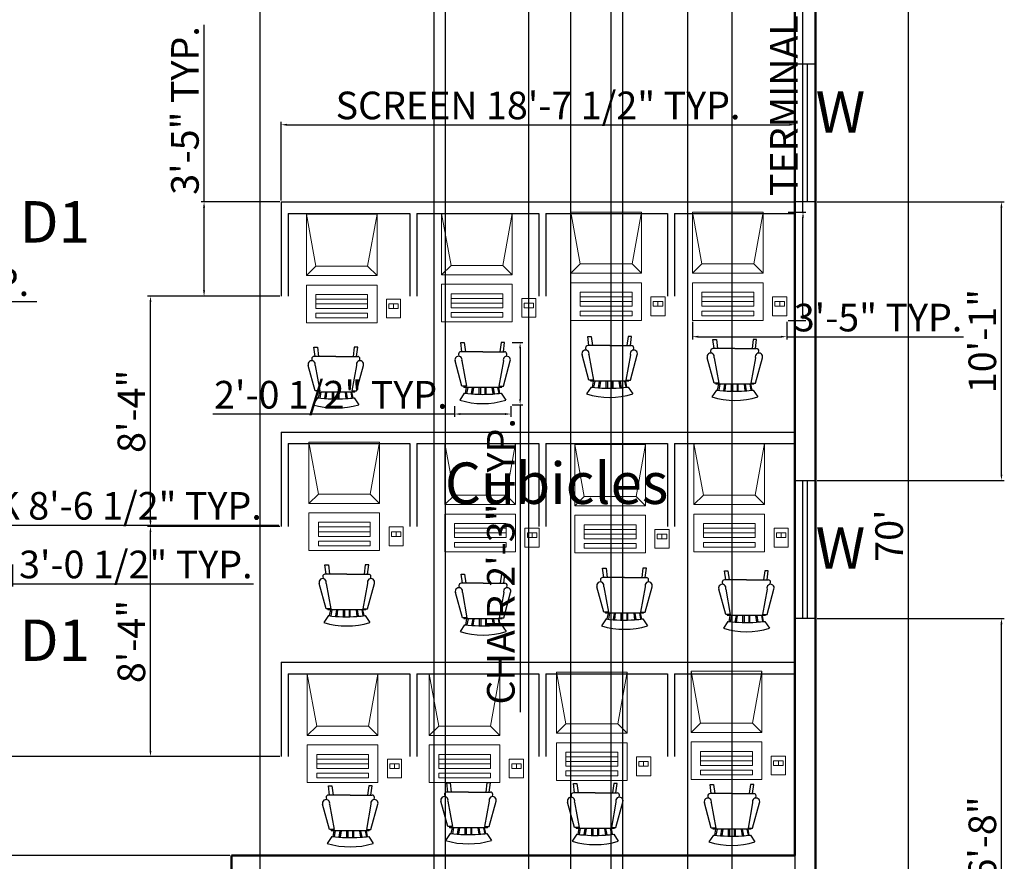
# Model space of a CAD drawing. Units: inches. Extents: x 1953 to 3378, y 1378 to 2530.
# Tile 3 of 5: x 2350 to 2778, y 1725 to 2090. Entities that reach past the tile are written whole.
import ezdxf

# ---------------------------------------------------------------- set-up
doc = ezdxf.new("R2010")
doc.units = ezdxf.units.IN
for name, color, linetype, lineweight in [('A-ANNO-DIMS', 2, 'Continuous', 18), ('A-ANNO-TEXT', 7, 'Continuous', 18), ('A-AREA-IDEN', 4, 'Continuous', 18), ('A-EQPM', 50, 'Continuous', 18), ('A-FURN', 50, 'Continuous', 25), ('wall', 7, 'Continuous', 50), ('windows', 180, 'Continuous', 25)]:
    doc.layers.add(name, color=color, linetype=linetype, lineweight=lineweight)
doc.styles.get("Standard").update_dxf_attribs({"font": 'arial.ttf'})
doc.dimstyles.new('ISO-25', dxfattribs={"dimtxt": 12, "dimasz": 2.5, "dimexe": 1.25, "dimexo": 0.625, "dimtad": 1, "dimdec": 1, "dimlunit": 4, "dimtxsty": 'Standard', "dimcen": 2.5, "dimadec": 0, "dimazin": 0, "dimtfac": 1, "dimtdec": 1, "dimtmove": 0, "dimatfit": 3, "dimfxl": 1, "dimarcsym": 0})

# ---------------------------------------------------------------- blocks, each defined once
blk = doc.blocks.new('Computer Terminal')
for p, q in [((-10, 11.5), (5, 11.5)), ((-8, 0.5), (-10, 11.5)), ((-10, -1.5), (-10, 11.5)), ((5, 11.5), (3, 0.5)), ((5, 11.5), (5, -1.5)), ((-10, -1.5), (-8, 0.5)), ((3, 0.5), (-8, 0.5)), ((3, 0.5), (5, -1.5)), ((5, -1.5), (-10, -1.5)), ((-10, -11.5), (-10, -3.5)), ((-10, -3.5), (5, -3.5)), ((5, -3.5), (5, -11.5)), ((-8, -5.5), (-8, -8.5)), ((3, -5.5), (-8, -5.5)), ((3, -8.5), (3, -5.5)), ((3, -6.5), (-8, -6.5)), ((-8, -7.5), (3, -7.5)), ((10, -6.5), (7, -6.5)), ((7, -6.5), (7, -10.5)), ((9.5, -7.5), (7.5, -7.5)), ((7.5, -7.5), (7.5, -8.5)), ((8.5, -7.5), (8.5, -8.5)), ((9.5, -8.5), (9.5, -7.5)), ((10, -10.5), (10, -6.5)), ((-8, -8.5), (3, -8.5)), ((-8, -9.5), (-8, -10.5)), ((3, -9.5), (-8, -9.5)), ((3, -10.5), (3, -9.5)), ((7.5, -8.5), (9.5, -8.5)), ((5, -11.5), (-10, -11.5)), ((-8, -10.5), (3, -10.5)), ((7, -10.5), (10, -10.5))]:
    blk.add_line(p, q)
blk = doc.blocks.new('Chair - Rocking')
for p, q in [((-8, -4.5), (-10, -1.5)), ((-4.5, -7), (-4.96674, -4.19951)), ((-4, -7), (-4.40532, -4.16272)), ((-1.5, -4.05012), (-1.5, -7)), ((-1, -7), (-1, -4.05012)), ((1, -7), (1, -4.04655)), ((1.5, -4.05012), (1.5, -7)), ((4, -7), (4.40187, -4.18694)), ((4.5, -7), (4.96761, -4.19437)), ((8, -4.5), (10, -1.5)), ((-9, -7.5), (-12, -18.49999)), ((-7, -7.5), (-9, -7.5)), ((-9, -18.49999), (-7, -7.5)), ((-8.23428, -6.99939), (-8.3093, -7.47958)), ((-8.23041, -7), (8.23915, -7)), ((-7.5, -4.5), (-7, -7)), ((-6.5, -7), (-7.02225, -4.43)), ((6.5, -7), (7, -4.4057)), ((7.5, -4.5), (7, -7)), ((7, -7.5), (9, -7.5)), ((9, -18.49999), (7, -7.5)), ((8.31071, -7.48854), (8.23449, -7.00073)), ((9, -7.5), (12, -18.49999)), ((-10.36644, -20.64523), (-10.5, -21.49999)), ((10.5, -21.49999), (10.3575, -20.58798)), ((-9, -22.49999), (-9.5, -26.49999)), ((0, -22.49999), (-9.5, -22.49999)), ((-8, -26.49999), (-7.5, -22.49999)), ((0, -22.49999), (9.5, -22.49999)), ((8, -26.49999), (7.5, -22.49999)), ((9, -22.49999), (9.5, -26.49999)), ((-9.5, -26.49999), (-8, -26.49999)), ((9.5, -26.49999), (8, -26.49999))]:
    blk.add_line(p, q)
for centre, radius, start, end in [((0, -34.08333), 34.08333, 72.93847, 107.0615), ((0, -68.25004), 64.25, 93.92211, 97.15267), ((0, -68.25004), 64.25, 82.84733, 93.92211), ((-10.5, -18.99999), 1.58114, 161.5651, 18.43495), ((10.5, -18.99999), 1.58114, 161.5651, 18.43495), ((-9.5, -21.49999), 1, 180, 270), ((9.5, -21.49999), 1, 270, 0)]:
    blk.add_arc(centre, radius, start, end)
blk = doc.blocks.new('*D27')
at = {"layer": 'A-ANNO-DIMS', "color": 0, "lineweight": -2, "transparency": 16777216}
for p, q in [((2696.37, 2286.01), (2737.23, 2286.01)), ((2735.98, 2283.51), (2735.98, 1448.51)), ((2696.37, 1446.01), (2737.23, 1446.01))]:
    blk.add_line(p, q, dxfattribs=at)
at = {"layer": 'A-ANNO-DIMS', "color": 0, "transparency": 16777216}
for points in [[(2735.56, 2283.51), (2736.4, 2283.51), (2735.98, 2286.01)], [(2735.56, 1448.51), (2736.4, 1448.51), (2735.98, 1446.01)]]:
    blk.add_solid(points, dxfattribs=at)
at = {"layer": 'Defpoints', "color": 0, "transparency": 16777216}
for p in [(2695.75, 2286.01), (2695.75, 1446.01), (2735.98, 1446.01)]:
    blk.add_point(p, dxfattribs=at)
at = {"layer": 'A-ANNO-DIMS', "color": 0, "transparency": 16777216, "insert": (2729.23, 1866.01), "char_height": 12, "attachment_point": 5, "rotation": 90}
blk.add_mtext("70'", dxfattribs=at)
blk = doc.blocks.new('WINDOW-60IN')
for p, q in [((0, 5.5), (60, 5.5)), ((0, 5.5), (60, 5.5)), ((0, 3.5), (60, 3.5))]:
    blk.add_line(p, q)
blk.add_lwpolyline([(0, 9), (60, 9), (60, 0), (0, 0)], close=True)
blk = doc.blocks.new('CUBICLE-SCREEN-4-BAY')
for p, q in [((0, 41), (223.35, 41)), ((0, 41), (0, 0)), ((3, 36), (56, 36)), ((3, 36), (3, 0)), ((56, 36), (56, 0)), ((59, 36), (59, 0)), ((59, 36), (112, 36)), ((112, 36), (112, 0)), ((115, 36), (115, 0)), ((115, 36), (168, 36)), ((168, 36), (168, 0)), ((171, 36), (171, 0)), ((171, 36), (223.35, 36))]:
    blk.add_line(p, q)
blk = doc.blocks.new('*D34')
at = {"layer": 'A-ANNO-DIMS', "color": 0, "lineweight": -2, "transparency": 16777216}
for p, q in [((2563.85, 1949.87), (2568.53, 1949.87)), ((2567.28, 1947.37), (2567.28, 1925.37)), ((2563.85, 1922.87), (2568.53, 1922.87)), ((2567.28, 1922.87), (2567.28, 1789.3))]:
    blk.add_line(p, q, dxfattribs=at)
at = {"layer": 'A-ANNO-DIMS', "color": 0, "transparency": 16777216}
for points in [[(2566.86, 1947.37), (2567.7, 1947.37), (2567.28, 1949.87)], [(2566.86, 1925.37), (2567.7, 1925.37), (2567.28, 1922.87)]]:
    blk.add_solid(points, dxfattribs=at)
at = {"layer": 'Defpoints', "color": 0, "transparency": 16777216}
for p in [(2563.23, 1949.87), (2563.23, 1922.87), (2567.28, 1922.87)]:
    blk.add_point(p, dxfattribs=at)
at = {"layer": 'A-ANNO-DIMS', "color": 0, "transparency": 16777216, "insert": (2560.44, 1854.83), "char_height": 12, "attachment_point": 5, "rotation": 90}
blk.add_mtext('CHAIR 2\'-3" TYP.', dxfattribs=at)
blk = doc.blocks.new('*D35')
at = {"layer": 'A-ANNO-DIMS', "color": 0, "lineweight": -2, "transparency": 16777216}
for p, q in [((2538.79, 1922.24), (2538.79, 1917.57)), ((2563.23, 1922.24), (2563.23, 1917.57)), ((2538.79, 1918.82), (2433.73, 1918.82)), ((2560.73, 1918.82), (2541.29, 1918.82))]:
    blk.add_line(p, q, dxfattribs=at)
at = {"layer": 'A-ANNO-DIMS', "color": 0, "transparency": 16777216}
for points in [[(2541.29, 1919.24), (2541.29, 1918.4), (2538.79, 1918.82)], [(2560.73, 1919.24), (2560.73, 1918.4), (2563.23, 1918.82)]]:
    blk.add_solid(points, dxfattribs=at)
at = {"layer": 'Defpoints', "color": 0, "transparency": 16777216}
for p in [(2538.79, 1922.87), (2563.23, 1922.87), (2538.79, 1918.82)]:
    blk.add_point(p, dxfattribs=at)
at = {"layer": 'A-ANNO-DIMS', "color": 0, "transparency": 16777216, "insert": (2485.01, 1925.65), "char_height": 12, "attachment_point": 5}
blk.add_mtext('2\'-0 1/2" TYP.', dxfattribs=at)
blk = doc.blocks.new('*D36')
at = {"layer": 'A-ANNO-DIMS', "color": 0, "lineweight": -2, "transparency": 16777216}
for p, q in [((2690.25, 2006.56), (2690.25, 2182.51)), ((2683.81, 2006.56), (2691.5, 2006.56)), ((2690.25, 1961.98), (2690.25, 2004.06)), ((2683.81, 1959.48), (2691.5, 1959.48))]:
    blk.add_line(p, q, dxfattribs=at)
at = {"layer": 'A-ANNO-DIMS', "color": 0, "transparency": 16777216}
for points in [[(2689.83, 2004.06), (2690.66, 2004.06), (2690.25, 2006.56)], [(2689.83, 1961.98), (2690.66, 1961.98), (2690.25, 1959.48)]]:
    blk.add_solid(points, dxfattribs=at)
at = {"layer": 'Defpoints', "color": 0, "transparency": 16777216}
for p in [(2683.18, 2006.56), (2690.25, 2006.56), (2683.18, 1959.48)]:
    blk.add_point(p, dxfattribs=at)
at = {"layer": 'A-ANNO-DIMS', "color": 0, "transparency": 16777216, "insert": (2683.49, 2095.79), "char_height": 12, "attachment_point": 5, "rotation": 90}
blk.add_mtext('TERMINAL 3\'-11" TYP.', dxfattribs=at)
blk = doc.blocks.new('*D37')
at = {"layer": 'A-ANNO-DIMS', "color": 0, "lineweight": -2, "transparency": 16777216}
for p, q in [((2642.24, 1958.85), (2642.24, 1951.16)), ((2683.18, 1958.85), (2683.18, 1951.16)), ((2644.74, 1952.41), (2680.68, 1952.41)), ((2683.18, 1952.41), (2760.07, 1952.41))]:
    blk.add_line(p, q, dxfattribs=at)
at = {"layer": 'A-ANNO-DIMS', "color": 0, "transparency": 16777216}
for points in [[(2644.74, 1952.83), (2644.74, 1952), (2642.24, 1952.41)], [(2680.68, 1952.83), (2680.68, 1952), (2683.18, 1952.41)]]:
    blk.add_solid(points, dxfattribs=at)
at = {"layer": 'Defpoints', "color": 0, "transparency": 16777216}
for p in [(2642.24, 1959.48), (2683.18, 1959.48), (2683.18, 1952.41)]:
    blk.add_point(p, dxfattribs=at)
at = {"layer": 'A-ANNO-DIMS', "color": 0, "transparency": 16777216, "insert": (2722.88, 1959.17), "char_height": 12, "attachment_point": 5}
blk.add_mtext('3\'-5" TYP.', dxfattribs=at)
blk = doc.blocks.new('*D41')
at = {"layer": 'A-ANNO-DIMS', "color": 0, "lineweight": -2, "transparency": 16777216}
for p, q in [((2309.89, 1853.46), (2309.89, 1843.84)), ((2346.56, 1853.46), (2346.56, 1843.84)), ((2312.39, 1845.09), (2344.06, 1845.09)), ((2346.56, 1845.09), (2451.41, 1845.09))]:
    blk.add_line(p, q, dxfattribs=at)
at = {"layer": 'A-ANNO-DIMS', "color": 0, "transparency": 16777216}
for points in [[(2312.39, 1845.5), (2312.39, 1844.67), (2309.89, 1845.09)], [(2344.06, 1845.5), (2344.06, 1844.67), (2346.56, 1845.09)]]:
    blk.add_solid(points, dxfattribs=at)
at = {"layer": 'Defpoints', "color": 0, "transparency": 16777216}
for p in [(2309.89, 1854.09), (2346.56, 1854.09), (2346.56, 1845.09)]:
    blk.add_point(p, dxfattribs=at)
at = {"layer": 'A-ANNO-DIMS', "color": 0, "transparency": 16777216, "insert": (2400.23, 1851.92), "char_height": 12, "attachment_point": 5}
blk.add_mtext('3\'-0 1/2" TYP.', dxfattribs=at)
blk = doc.blocks.new('*D42')
at = {"layer": 'A-ANNO-DIMS', "color": 0, "lineweight": -2, "transparency": 16777216}
for p, q in [((2146.13, 1979.72), (2146.13, 1966.49)), ((2230.13, 1979.72), (2230.13, 1966.49)), ((2148.63, 1967.74), (2227.63, 1967.74)), ((2230.13, 1967.74), (2357.26, 1967.74))]:
    blk.add_line(p, q, dxfattribs=at)
at = {"layer": 'A-ANNO-DIMS', "color": 0, "transparency": 16777216}
for points in [[(2148.63, 1968.16), (2148.63, 1967.33), (2146.13, 1967.74)], [(2227.63, 1968.16), (2227.63, 1967.33), (2230.13, 1967.74)]]:
    blk.add_solid(points, dxfattribs=at)
at = {"layer": 'Defpoints', "color": 0, "transparency": 16777216}
for p in [(2146.13, 1980.34), (2230.13, 1980.34), (2230.13, 1967.74)]:
    blk.add_point(p, dxfattribs=at)
at = {"layer": 'A-ANNO-DIMS', "color": 0, "transparency": 16777216, "insert": (2294.95, 1974.58), "char_height": 12, "attachment_point": 5}
blk.add_mtext('SOFA 7\'-0" TYP.', dxfattribs=at)
blk = doc.blocks.new('*D44')
at = {"layer": 'A-ANNO-DIMS', "color": 0, "lineweight": -2, "transparency": 16777216}
for p, q in [((2129.36, 1885.33), (2129.36, 1869.31)), ((2231.98, 1885.33), (2231.98, 1869.31)), ((2131.86, 1870.56), (2229.48, 1870.56)), ((2231.98, 1870.56), (2462.45, 1870.56))]:
    blk.add_line(p, q, dxfattribs=at)
at = {"layer": 'A-ANNO-DIMS', "color": 0, "transparency": 16777216}
for points in [[(2131.86, 1870.98), (2131.86, 1870.14), (2129.36, 1870.56)], [(2229.48, 1870.98), (2229.48, 1870.14), (2231.98, 1870.56)]]:
    blk.add_solid(points, dxfattribs=at)
at = {"layer": 'Defpoints', "color": 0, "transparency": 16777216}
for p in [(2129.36, 1885.95), (2231.98, 1885.95), (2231.98, 1870.56)]:
    blk.add_point(p, dxfattribs=at)
at = {"layer": 'A-ANNO-DIMS', "color": 0, "transparency": 16777216, "insert": (2348.46, 1877.39), "char_height": 12, "attachment_point": 5}
blk.add_mtext('CURVED DESK 8\'-6 1/2" TYP.', dxfattribs=at)
blk = doc.blocks.new('*D46')
at = {"layer": 'A-ANNO-DIMS', "color": 0, "lineweight": -2, "transparency": 16777216}
for p, q in [((2463.39, 2011.62), (2463.39, 2045.75)), ((2465.89, 2044.5), (2684.25, 2044.5)), ((2686.75, 2011.62), (2686.75, 2045.75))]:
    blk.add_line(p, q, dxfattribs=at)
at = {"layer": 'A-ANNO-DIMS', "color": 0, "transparency": 16777216}
for points in [[(2465.89, 2044.92), (2465.89, 2044.09), (2463.39, 2044.5)], [(2684.25, 2044.92), (2684.25, 2044.09), (2686.75, 2044.5)]]:
    blk.add_solid(points, dxfattribs=at)
at = {"layer": 'Defpoints', "color": 0, "transparency": 16777216}
for p in [(2686.75, 2044.5), (2463.39, 2011), (2686.75, 2011)]:
    blk.add_point(p, dxfattribs=at)
at = {"layer": 'A-ANNO-DIMS', "color": 0, "transparency": 16777216, "insert": (2575.07, 2051.33), "char_height": 12, "attachment_point": 5}
blk.add_mtext('SCREEN 18\'-7 1/2" TYP.', dxfattribs=at)
blk = doc.blocks.new('*D47')
at = {"layer": 'A-ANNO-DIMS', "color": 0, "lineweight": -2, "transparency": 16777216}
for p, q in [((2429.89, 2011), (2429.89, 2087.89)), ((2462.77, 2011), (2428.64, 2011)), ((2429.89, 1972.5), (2429.89, 2008.5)), ((2462.77, 1970), (2428.64, 1970))]:
    blk.add_line(p, q, dxfattribs=at)
at = {"layer": 'A-ANNO-DIMS', "color": 0, "transparency": 16777216}
for points in [[(2429.47, 2008.5), (2430.31, 2008.5), (2429.89, 2011)], [(2429.47, 1972.5), (2430.31, 1972.5), (2429.89, 1970)]]:
    blk.add_solid(points, dxfattribs=at)
at = {"layer": 'Defpoints', "color": 0, "transparency": 16777216}
for p in [(2429.89, 2011), (2463.39, 2011), (2463.39, 1970)]:
    blk.add_point(p, dxfattribs=at)
at = {"layer": 'A-ANNO-DIMS', "color": 0, "transparency": 16777216, "insert": (2423.13, 2050.69), "char_height": 12, "attachment_point": 5, "rotation": 90}
blk.add_mtext('3\'-5" TYP.', dxfattribs=at)
blk = doc.blocks.new('*D64')
at = {"layer": 'A-ANNO-DIMS', "color": 0, "lineweight": -2, "transparency": 16777216}
for p, q in [((2462.77, 1870), (2405.34, 1870)), ((2406.59, 1772.5), (2406.59, 1867.5)), ((2462.77, 1770), (2405.34, 1770))]:
    blk.add_line(p, q, dxfattribs=at)
at = {"layer": 'A-ANNO-DIMS', "color": 0, "transparency": 16777216}
for points in [[(2406.18, 1867.5), (2407.01, 1867.5), (2406.59, 1870)], [(2406.18, 1772.5), (2407.01, 1772.5), (2406.59, 1770)]]:
    blk.add_solid(points, dxfattribs=at)
at = {"layer": 'Defpoints', "color": 0, "transparency": 16777216}
for p in [(2406.59, 1870), (2463.39, 1870), (2463.39, 1770)]:
    blk.add_point(p, dxfattribs=at)
at = {"layer": 'A-ANNO-DIMS', "color": 0, "transparency": 16777216, "insert": (2399.84, 1820), "char_height": 12, "attachment_point": 5, "rotation": 90}
blk.add_mtext('8\'-4"', dxfattribs=at)
blk = doc.blocks.new('*D65')
at = {"layer": 'A-ANNO-DIMS', "color": 0, "lineweight": -2, "transparency": 16777216}
for p, q in [((2462.77, 1970), (2405.34, 1970)), ((2406.59, 1872.5), (2406.59, 1967.5)), ((2462.77, 1870), (2405.34, 1870))]:
    blk.add_line(p, q, dxfattribs=at)
at = {"layer": 'A-ANNO-DIMS', "color": 0, "transparency": 16777216}
for points in [[(2406.18, 1967.5), (2407.01, 1967.5), (2406.59, 1970)], [(2406.18, 1872.5), (2407.01, 1872.5), (2406.59, 1870)]]:
    blk.add_solid(points, dxfattribs=at)
at = {"layer": 'Defpoints', "color": 0, "transparency": 16777216}
for p in [(2406.59, 1970), (2463.39, 1970), (2463.39, 1870)]:
    blk.add_point(p, dxfattribs=at)
at = {"layer": 'A-ANNO-DIMS', "color": 0, "transparency": 16777216, "insert": (2399.84, 1920), "char_height": 12, "attachment_point": 5, "rotation": 90}
blk.add_mtext('8\'-4"', dxfattribs=at)
blk = doc.blocks.new('*D72')
at = {"layer": 'A-ANNO-DIMS', "color": 0, "lineweight": -2, "transparency": 16777216}
for p, q in [((2696.37, 1830.01), (2777.76, 1830.01)), ((2776.51, 1632.66), (2776.51, 1827.51)), ((2696.37, 1630.16), (2777.76, 1630.16))]:
    blk.add_line(p, q, dxfattribs=at)
at = {"layer": 'A-ANNO-DIMS', "color": 0, "transparency": 16777216}
for points in [[(2776.09, 1827.51), (2776.93, 1827.51), (2776.51, 1830.01)], [(2776.09, 1632.66), (2776.93, 1632.66), (2776.51, 1630.16)]]:
    blk.add_solid(points, dxfattribs=at)
at = {"layer": 'Defpoints', "color": 0, "transparency": 16777216}
for p in [(2695.75, 1830.01), (2776.51, 1830.01), (2695.75, 1630.16)]:
    blk.add_point(p, dxfattribs=at)
at = {"layer": 'A-ANNO-DIMS', "color": 0, "transparency": 16777216, "insert": (2769.76, 1730.09), "char_height": 12, "attachment_point": 5, "rotation": 90}
blk.add_mtext('16\'-8"', dxfattribs=at)
blk = doc.blocks.new('*D73')
at = {"layer": 'A-ANNO-DIMS', "color": 0, "lineweight": -2, "transparency": 16777216}
for p, q in [((2696.37, 2011), (2777.76, 2011)), ((2776.51, 1892.51), (2776.51, 2008.5)), ((2696.37, 1890.01), (2777.76, 1890.01))]:
    blk.add_line(p, q, dxfattribs=at)
at = {"layer": 'A-ANNO-DIMS', "color": 0, "transparency": 16777216}
for points in [[(2776.09, 2008.5), (2776.93, 2008.5), (2776.51, 2011)], [(2776.09, 1892.51), (2776.93, 1892.51), (2776.51, 1890.01)]]:
    blk.add_solid(points, dxfattribs=at)
at = {"layer": 'Defpoints', "color": 0, "transparency": 16777216}
for p in [(2695.75, 2011), (2776.51, 2011), (2695.75, 1890.01)]:
    blk.add_point(p, dxfattribs=at)
at = {"layer": 'A-ANNO-DIMS', "color": 0, "transparency": 16777216, "insert": (2769.76, 1950.51), "char_height": 12, "attachment_point": 5, "rotation": 90}
blk.add_mtext('10\'-1"', dxfattribs=at)
blk = doc.blocks.new('*D74')
at = {"layer": 'A-ANNO-DIMS', "color": 0, "lineweight": -2, "transparency": 16777216}
for p, q in [((2454.07, 2276.39), (2454.07, 1387.78)), ((2529.75, 2276.39), (2529.75, 1387.78)), ((2456.57, 1389.03), (2527.25, 1389.03))]:
    blk.add_line(p, q, dxfattribs=at)
at = {"layer": 'A-ANNO-DIMS', "color": 0, "transparency": 16777216}
for points in [[(2456.57, 1389.45), (2456.57, 1388.62), (2454.07, 1389.03)], [(2527.25, 1389.45), (2527.25, 1388.62), (2529.75, 1389.03)]]:
    blk.add_solid(points, dxfattribs=at)
at = {"layer": 'Defpoints', "color": 0, "transparency": 16777216}
for p in [(2454.07, 2277.01), (2529.75, 2277.01), (2529.75, 1389.03)]:
    blk.add_point(p, dxfattribs=at)
at = {"layer": 'A-ANNO-DIMS', "color": 0, "transparency": 16777216, "insert": (2491.91, 1395.87), "char_height": 12, "attachment_point": 5}
blk.add_mtext('6\'-3 1/2"', dxfattribs=at)
blk = doc.blocks.new('*D80')
at = {"layer": 'A-ANNO-DIMS', "color": 0, "lineweight": -2, "transparency": 16777216}
for p, q in [((2534.75, 2161.39), (2534.75, 1387.78)), ((2570.9, 2161.44), (2570.9, 1387.78)), ((2537.25, 1389.03), (2568.4, 1389.03))]:
    blk.add_line(p, q, dxfattribs=at)
at = {"layer": 'A-ANNO-DIMS', "color": 0, "transparency": 16777216}
for points in [[(2537.25, 1389.45), (2537.25, 1388.62), (2534.75, 1389.03)], [(2568.4, 1389.45), (2568.4, 1388.62), (2570.9, 1389.03)]]:
    blk.add_solid(points, dxfattribs=at)
at = {"layer": 'Defpoints', "color": 0, "transparency": 16777216}
for p in [(2534.75, 2162.01), (2570.9, 2162.07), (2570.9, 1389.03)]:
    blk.add_point(p, dxfattribs=at)
at = {"layer": 'A-ANNO-DIMS', "color": 0, "transparency": 16777216, "insert": (2552.82, 1395.79), "char_height": 12, "attachment_point": 5}
blk.add_mtext('3\'-0"', dxfattribs=at)
blk = doc.blocks.new('*D81')
at = {"layer": 'A-ANNO-DIMS', "color": 0, "lineweight": -2, "transparency": 16777216}
for p, q in [((2659.25, 2159.09), (2659.25, 1387.78)), ((2686.75, 2161.39), (2686.75, 1387.78)), ((2661.75, 1389.03), (2684.25, 1389.03)), ((2686.75, 1389.03), (2750.56, 1389.03))]:
    blk.add_line(p, q, dxfattribs=at)
at = {"layer": 'A-ANNO-DIMS', "color": 0, "transparency": 16777216}
for points in [[(2661.75, 1389.45), (2661.75, 1388.62), (2659.25, 1389.03)], [(2684.25, 1389.45), (2684.25, 1388.62), (2686.75, 1389.03)]]:
    blk.add_solid(points, dxfattribs=at)
at = {"layer": 'Defpoints', "color": 0, "transparency": 16777216}
for p in [(2686.75, 2162.01), (2659.25, 2159.71), (2686.75, 1389.03)]:
    blk.add_point(p, dxfattribs=at)
at = {"layer": 'A-ANNO-DIMS', "color": 0, "transparency": 16777216, "insert": (2719.91, 1395.87), "char_height": 12, "attachment_point": 5}
blk.add_mtext('2\'-3 1/2"', dxfattribs=at)
blk = doc.blocks.new('*D82')
at = {"layer": 'A-ANNO-DIMS', "color": 0, "lineweight": -2, "transparency": 16777216}
for p, q in [((2606.75, 2161.39), (2606.75, 1387.78)), ((2611.75, 2161.39), (2611.75, 1387.78)), ((2604.25, 1389.03), (2601.75, 1389.03)), ((2606.75, 1389.03), (2611.75, 1389.03)), ((2614.25, 1389.03), (2649.9, 1389.03))]:
    blk.add_line(p, q, dxfattribs=at)
at = {"layer": 'A-ANNO-DIMS', "color": 0, "transparency": 16777216}
for points in [[(2604.25, 1389.45), (2604.25, 1388.62), (2606.75, 1389.03)], [(2614.25, 1389.45), (2614.25, 1388.62), (2611.75, 1389.03)]]:
    blk.add_solid(points, dxfattribs=at)
at = {"layer": 'Defpoints', "color": 0, "transparency": 16777216}
for p in [(2606.75, 2162.01), (2611.75, 2162.01), (2611.75, 1389.03)]:
    blk.add_point(p, dxfattribs=at)
at = {"layer": 'A-ANNO-DIMS', "color": 0, "transparency": 16777216, "insert": (2633.32, 1395.79), "char_height": 12, "attachment_point": 5}
blk.add_mtext('0\'-5"', dxfattribs=at)
blk = doc.blocks.new('*D83')
at = {"layer": 'A-ANNO-DIMS', "color": 0, "lineweight": -2, "transparency": 16777216}
for p, q in [((2462.77, 1770), (1976.77, 1770)), ((1978.02, 1729.51), (1978.02, 1767.5)), ((2441.12, 1727.01), (1976.77, 1727.01))]:
    blk.add_line(p, q, dxfattribs=at)
at = {"layer": 'A-ANNO-DIMS', "color": 0, "transparency": 16777216}
for points in [[(1977.6, 1767.5), (1978.44, 1767.5), (1978.02, 1770)], [(1977.6, 1729.51), (1978.44, 1729.51), (1978.02, 1727.01)]]:
    blk.add_solid(points, dxfattribs=at)
at = {"layer": 'Defpoints', "color": 0, "transparency": 16777216}
for p in [(1978.02, 1770), (2463.39, 1770), (2441.75, 1727.01)]:
    blk.add_point(p, dxfattribs=at)
at = {"layer": 'A-ANNO-DIMS', "color": 0, "transparency": 16777216, "insert": (1971.26, 1748.51), "char_height": 12, "attachment_point": 5, "rotation": 90}
blk.add_mtext('3\'-7"', dxfattribs=at)
blk = doc.blocks.new('*D84')
at = {"layer": 'A-ANNO-DIMS', "color": 0, "lineweight": -2, "transparency": 16777216}
for p, q in [((2606.75, 2276.39), (2606.75, 1387.78)), ((2589.14, 2267.41), (2589.14, 1387.78)), ((2591.64, 1389.03), (2604.25, 1389.03)), ((2606.75, 1389.03), (2669.23, 1389.03))]:
    blk.add_line(p, q, dxfattribs=at)
at = {"layer": 'A-ANNO-DIMS', "color": 0, "transparency": 16777216}
for points in [[(2591.64, 1389.45), (2591.64, 1388.62), (2589.14, 1389.03)], [(2604.25, 1389.45), (2604.25, 1388.62), (2606.75, 1389.03)]]:
    blk.add_solid(points, dxfattribs=at)
at = {"layer": 'Defpoints', "color": 0, "transparency": 16777216}
for p in [(2606.75, 2277.01), (2589.14, 2268.03), (2606.75, 1389.03)]:
    blk.add_point(p, dxfattribs=at)
at = {"layer": 'A-ANNO-DIMS', "color": 0, "transparency": 16777216, "insert": (2639.24, 1395.86), "char_height": 12, "attachment_point": 5}
blk.add_mtext('1\'-5 1/2"', dxfattribs=at)
blk = doc.blocks.new('*D85')
at = {"layer": 'A-ANNO-DIMS', "color": 0, "lineweight": -2, "transparency": 16777216}
for p, q in [((2611.75, 2276.39), (2611.75, 1387.78)), ((2640.05, 2268.38), (2640.05, 1387.78)), ((2614.25, 1389.03), (2637.55, 1389.03)), ((2640.05, 1389.03), (2703.87, 1389.03))]:
    blk.add_line(p, q, dxfattribs=at)
at = {"layer": 'A-ANNO-DIMS', "color": 0, "transparency": 16777216}
for points in [[(2614.25, 1389.45), (2614.25, 1388.62), (2611.75, 1389.03)], [(2637.55, 1389.45), (2637.55, 1388.62), (2640.05, 1389.03)]]:
    blk.add_solid(points, dxfattribs=at)
at = {"layer": 'Defpoints', "color": 0, "transparency": 16777216}
for p in [(2611.75, 2277.01), (2640.05, 2269), (2640.05, 1389.03)]:
    blk.add_point(p, dxfattribs=at)
at = {"layer": 'A-ANNO-DIMS', "color": 0, "transparency": 16777216, "insert": (2673.21, 1395.86), "char_height": 12, "attachment_point": 5}
blk.add_mtext('2\'-4 1/2"', dxfattribs=at)

msp = doc.modelspace()

# ---------------------------------------------------------------- linework, layer by layer
at = {"layer": 'wall'}
for p, q in [((2695.75, 2286.01), (2695.75, 1446.01)), ((2686.75, 2157.01), (2686.75, 2011)), ((2686.75, 2011), (2686.75, 1806)), ((2686.75, 1830.01), (2686.75, 1811)), ((2686.75, 1806), (2686.75, 1727.01)), ((2686.75, 1806), (2686.75, 1727.01)), ((2441.75, 1727.01), (2686.75, 1727.01)), ((2441.75, 1727.01), (2441.75, 1455.01))]:
    msp.add_line(p, q, dxfattribs=at)

# ---------------------------------------------------------------- block references
at = {"layer": 'A-EQPM', "xscale": 2.047281239074101, "yscale": 2.047281239074101, "zscale": 2.047281239074101}
for p in [(2494.86, 1982.04), (2553.64, 1982.37), (2609.81, 1983.02), (2662.71, 1983.02), (2495.97, 1883.05), (2555.07, 1882.52), (2611.55, 1882), (2663.33, 1882.52), (2603.56, 1783.2), (2662.13, 1783.52), (2495.25, 1782.22), (2548.26, 1782.22)]:
    msp.add_blockref('Computer Terminal', p, dxfattribs=at)
at = {"layer": 'A-FURN'}
for p in [(2463.39, 1970), (2463.39, 1870), (2463.39, 1770)]:
    msp.add_blockref('CUBICLE-SCREEN-4-BAY', p, dxfattribs=at)
at = {"layer": 'A-FURN', "rotation": 180}
for p in [(2606.21, 1926.03), (2487.17, 1921.38), (2551.01, 1923.37), (2660.61, 1924.73), (2491.96, 1826.74), (2551.17, 1822.79), (2612.66, 1825.29), (2665.64, 1824.26), (2493.45, 1730.78), (2544.86, 1732.08), (2599.95, 1731.75), (2659.37, 1731.42)]:
    msp.add_blockref('Chair - Rocking', p, dxfattribs=at)
at = {"layer": 'windows'}
for p, rotation in [((2695.75, 2011), 90.00000000000063), ((2695.75, 1830.01), 90.00000000000072)]:
    msp.add_blockref('WINDOW-60IN', p, dxfattribs=dict(at, rotation=rotation))

# ---------------------------------------------------------------- texts
at = {"layer": 'A-ANNO-TEXT'}
for s, p in [('W', (2695.75, 2041)), ('D1', (2349.75, 1993.32)), ('W', (2695.75, 1851.59)), ('D1', (2349.75, 1811.55))]:
    msp.add_text(s, height=18, dxfattribs=at).set_placement(p)
at = {"layer": 'A-AREA-IDEN'}
msp.add_text('Cubicles', height=18, dxfattribs=at).set_placement((2534.6, 1879.76))

# ---------------------------------------------------------------- dimensions: what is measured, and where the dimension line sits
at = {"layer": 'A-ANNO-DIMS'}
for base, p1, p2, override, picture, middle in [((2735.98, 1446.01), (2695.75, 2286.01), (2695.75, 1446.01), {"dimclrd": 0, "dimclre": 0, "dimclrt": 0}, '*D27', (2729.23, 1866.01)), ((2776.51, 2011), (2695.75, 1890.01), (2695.75, 2011), {"dimdec": 1, "dimlfac": 1, "dimrnd": 0, "dimzin": 1, "dimdsep": 46, "dimlunit": 4, "dimfrac": 2}, '*D73', (2769.76, 1950.51)), ((2406.59, 1970), (2463.39, 1870), (2463.39, 1970), {"dimdec": 1, "dimlfac": 1, "dimrnd": 0, "dimzin": 1, "dimdsep": 46, "dimlunit": 4, "dimfrac": 2}, '*D65', (2399.84, 1920)), ((2406.59, 1870), (2463.39, 1770), (2463.39, 1870), {"dimdec": 1, "dimlfac": 1, "dimrnd": 0, "dimzin": 1, "dimdsep": 46, "dimlunit": 4, "dimfrac": 2}, '*D64', (2399.84, 1820)), ((2776.5098, 1830.0108), (2695.7476, 1630.1645), (2695.7476, 1830.0108), {"dimdec": 1, "dimlfac": 1, "dimrnd": 0, "dimzin": 1, "dimdsep": 46, "dimlunit": 4, "dimfrac": 2}, '*D72', (2769.758, 1730.0877)), ((1978.02, 1770), (2441.75, 1727.01), (2463.39, 1770), {"dimdec": 1, "dimlfac": 1, "dimrnd": 0, "dimzin": 1, "dimdsep": 46, "dimlunit": 4, "dimfrac": 2}, '*D83', (1971.26, 1748.51))]:
    dim = msp.add_linear_dim(base=base, p1=p1, p2=p2, angle=90, dimstyle='ISO-25', override=override, dxfattribs=at)
    dim.commit()
    dim.dimension.update_dxf_attribs({"geometry": picture, "text_midpoint": middle})
for base, p1, p2, picture, middle in [((2529.75, 1389.03), (2454.07, 2277.01), (2529.75, 2277.01), '*D74', (2491.91, 1395.87)), ((2606.75, 1389.03), (2589.14, 2268.03), (2606.75, 2277.01), '*D84', (2639.24, 1395.86)), ((2640.05, 1389.03), (2611.75, 2277.01), (2640.05, 2269), '*D85', (2673.21, 1395.86)), ((2570.9022, 1389.0336), (2534.7476, 2162.0108), (2570.9022, 2162.0653), '*D80', (2552.8249, 1395.7895)), ((2611.75, 1389.03), (2606.75, 2162.01), (2611.75, 2162.01), '*D82', (2633.32, 1395.79)), ((2686.75, 1389.03), (2659.25, 2159.71), (2686.75, 2162.01), '*D81', (2719.91, 1395.87))]:
    dim = msp.add_linear_dim(base=base, p1=p1, p2=p2, dimstyle='ISO-25', override={"dimdec": 1, "dimlfac": 1, "dimrnd": 0, "dimzin": 1, "dimdsep": 46, "dimlunit": 4, "dimfrac": 2}, dxfattribs=at)
    dim.commit()
    dim.dimension.update_dxf_attribs({"geometry": picture, "text_midpoint": middle})
for base, p1, p2, angle, text, picture, middle in [((2690.25, 2006.56), (2683.18, 1959.48), (2683.18, 2006.56), 90, 'TERMINAL <> TYP.', '*D36', (2683.49, 2095.79)), ((2429.89, 2011), (2463.39, 1970), (2463.39, 2011), 90, '<> TYP.', '*D47', (2423.13, 2050.69)), ((2538.79, 1918.82), (2563.23, 1922.87), (2538.79, 1922.87), 180, '<> TYP.', '*D35', (2485.01, 1925.65)), ((2567.28, 1922.87), (2563.23, 1949.87), (2563.23, 1922.87), 270, 'CHAIR <> TYP.', '*D34', (2560.44, 1854.83))]:
    dim = msp.add_linear_dim(base=base, p1=p1, p2=p2, angle=angle, text=text, dimstyle='ISO-25', override={"dimdec": 1, "dimlfac": 1, "dimrnd": 0, "dimzin": 1, "dimdsep": 46, "dimlunit": 4, "dimfrac": 2}, dxfattribs=at)
    dim.commit()
    dim.dimension.update_dxf_attribs({"geometry": picture, "text_midpoint": middle})
for base, p1, p2, text, picture, middle in [((2686.75, 2044.5), (2463.39, 2011), (2686.75, 2011), 'SCREEN <> TYP.', '*D46', (2575.07, 2051.33)), ((2230.13, 1967.74), (2146.13, 1980.34), (2230.13, 1980.34), 'SOFA <> TYP.', '*D42', (2294.95, 1974.58)), ((2683.18, 1952.41), (2642.24, 1959.48), (2683.18, 1959.48), '<> TYP.', '*D37', (2722.88, 1959.17)), ((2231.98, 1870.56), (2129.36, 1885.95), (2231.98, 1885.95), 'CURVED DESK <> TYP.', '*D44', (2348.46, 1877.39)), ((2346.56, 1845.09), (2309.89, 1854.09), (2346.56, 1854.09), '<> TYP.', '*D41', (2400.23, 1851.92))]:
    dim = msp.add_linear_dim(base=base, p1=p1, p2=p2, text=text, dimstyle='ISO-25', override={"dimdec": 1, "dimlfac": 1, "dimrnd": 0, "dimzin": 1, "dimdsep": 46, "dimlunit": 4, "dimfrac": 2}, dxfattribs=at)
    dim.commit()
    dim.dimension.update_dxf_attribs({"geometry": picture, "text_midpoint": middle})

doc.saveas('drawing.dxf')
